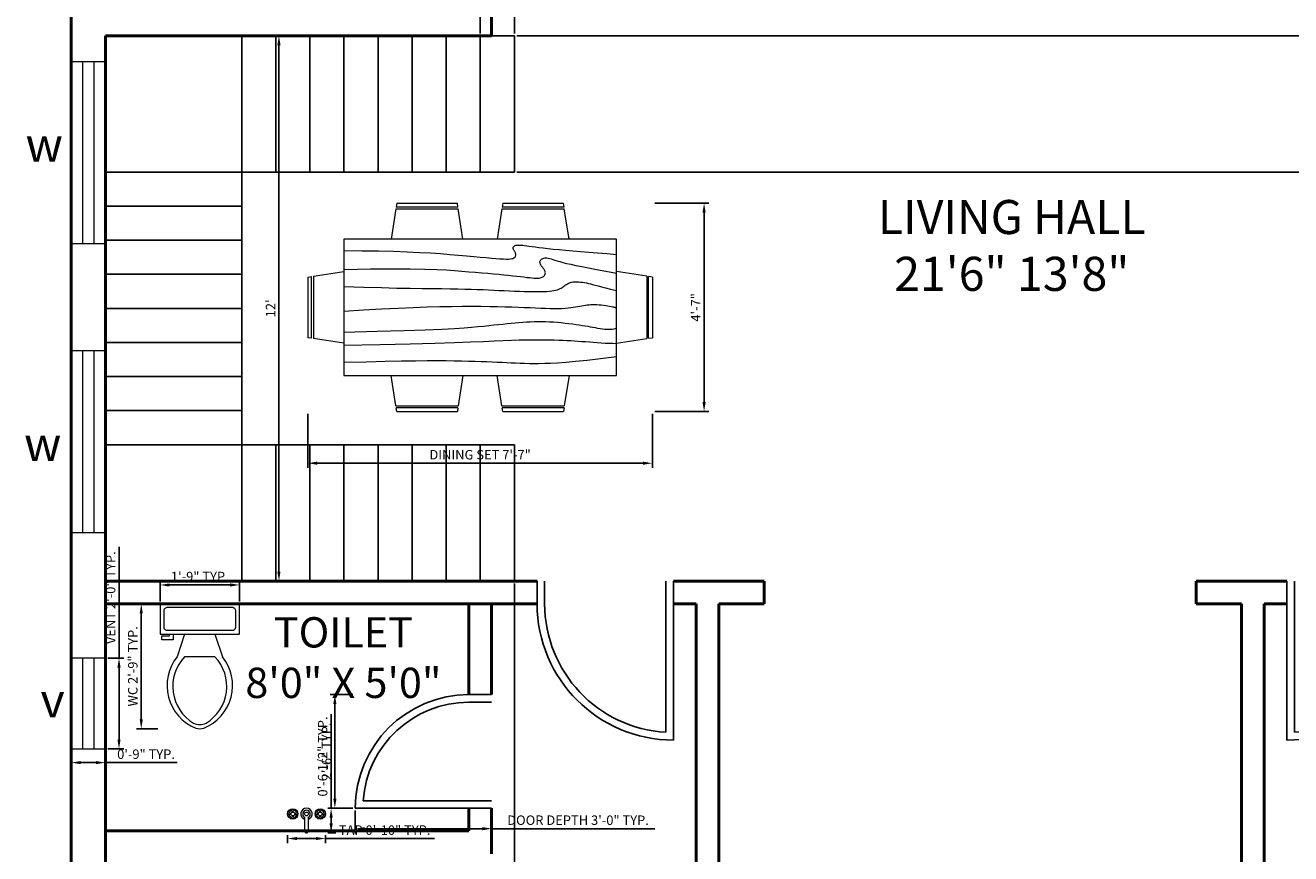
# Model space of a CAD drawing. Units: inches. Extents: x 1776 to 2338, y 1299 to 2099.
# Tile 2 of 4: x 1807 to 2141, y 1617 to 1836. Entities that reach past the tile are written whole.
import ezdxf

# ---------------------------------------------------------------- set-up
doc = ezdxf.new("R2010")
doc.units = ezdxf.units.IN
for name, color, linetype, lineweight in [('A-ANNO-DIMS', 2, 'Continuous', 18), ('A-ANNO-TEXT', 7, 'Continuous', 18), ('A-AREA-IDEN', 7, 'Continuous', 25), ('A-DOOR', 4, 'Continuous', 25), ('A-FLOR-FIXT', 9, 'Continuous', 18), ('A-FLOR-STRS', 7, 'Continuous', 25), ('A-FURN', 8, 'Continuous', 18), ('A-GLAZ', 4, 'Continuous', 18), ('A-WALL', 7, 'Continuous', 50)]:
    doc.layers.add(name, color=color, linetype=linetype, lineweight=lineweight)
doc.styles.get("Standard").update_dxf_attribs({"font": 'arial.ttf'})
doc.dimstyles.new('ISO-25', dxfattribs={"dimtxt": 2.5, "dimasz": 2.5, "dimexe": 1.25, "dimexo": 0.625, "dimtad": 1, "dimdec": 0, "dimlunit": 3, "dimtxsty": 'Standard', "dimcen": 2.5, "dimadec": 0, "dimazin": 0, "dimtfac": 1, "dimtdec": 0, "dimtmove": 0, "dimatfit": 3, "dimfxl": 1, "dimarcsym": 0})

# ---------------------------------------------------------------- blocks, each defined once
blk = doc.blocks.new('Dining Set - 36 x 72 in.')
for p, q in [((-22, 27.5), (-22.1562, 26.50042)), ((-22, 27.5), (-6, 27.5)), ((-5.8437, 26.49966), (-6, 27.5)), ((6, 27.5), (5.8438, 26.50042)), ((6, 27.5), (22, 27.5)), ((22.1563, 26.49966), (22, 27.5)), ((-22.2343, 26.00059), (-23.4847, 17.99762)), ((-22.2304, 26), (-5.7608, 26)), ((-5.8416, 26.5), (-22.1534, 26.5)), ((-4.5152, 17.99762), (-5.7655, 25.99926)), ((5.7657, 26.00059), (4.5153, 17.99762)), ((5.7696, 26), (22.2392, 26)), ((22.1584, 26.5), (5.8466, 26.5)), ((23.4848, 17.99762), (22.2345, 25.99926)), ((36, 18), (-36, 18)), ((-36, 18), (-36, -18)), ((36, -18), (36, 18)), ((-45.5, 8), (-44.5004, 8.15617)), ((-45.5, 8), (-45.5, -8)), ((-44.5, -8.15843), (-44.5, 8.15338)), ((-44.0006, 8.23428), (-35.9976, 9.48474)), ((-44, 8.23041), (-44, -8.23915)), ((44.0006, 8.23428), (35.9976, 9.48474)), ((44, 8.23041), (44, -8.23915)), ((44.5, -8.15843), (44.5, 8.15338)), ((45.5, 8), (44.5005, 8.15617)), ((45.5, 8), (45.5, -8)), ((-44.4997, -8.15631), (-45.5, -8)), ((-35.9976, -9.48476), (-43.9993, -8.2345)), ((35.9976, -9.48476), (43.9993, -8.2345)), ((44.4997, -8.15631), (45.5, -8)), ((-36, -18), (36, -18)), ((-22.2343, -26.0006), (-23.4847, -17.99762)), ((-4.5152, -17.99762), (-5.7655, -25.99928)), ((5.7657, -26.0006), (4.5153, -17.99762)), ((23.4848, -17.99762), (22.2345, -25.99928)), ((-22.2304, -26), (-5.7608, -26)), ((-22, -27.5), (-22.1562, -26.50044)), ((-5.8416, -26.5), (-22.1534, -26.5)), ((-5.8437, -26.49967), (-6, -27.5)), ((5.7696, -26), (22.2392, -26)), ((6, -27.5), (5.8438, -26.50044)), ((22.1584, -26.5), (5.8466, -26.5)), ((22.1563, -26.49967), (22, -27.5)), ((-22, -27.5), (-6, -27.5)), ((6, -27.5), (22, -27.5))]:
    blk.add_line(p, q)
for points in [[(-36, 15), (-31.1772, 14.97754), (-26.8079, 14.91406), (-22.8538, 14.81543), (-19.276, 14.6875), (-16.0362, 14.53613), (-13.0957, 14.36718), (-10.4159, 14.18652), (-7.9583, 14), (-5.6904, 13.81315), (-3.6035, 13.63021), (-1.6954, 13.45508), (0.0365, 13.29166), (1.5945, 13.14388), (2.9811, 13.01562), (4.1988, 12.9108), (5.25, 12.83333), (6.1393, 12.78613), (6.8802, 12.76823), (7.4883, 12.77767), (7.9792, 12.8125), (8.3685, 12.87077), (8.6719, 12.95052), (8.9049, 13.0498), (9.0833, 13.16666), (9.2205, 13.29899), (9.3216, 13.44401), (9.3895, 13.59879), (9.4271, 13.76041), (9.4373, 13.92594), (9.4232, 14.09245), (9.3875, 14.257), (9.3333, 14.41666), (9.2638, 14.56917), (9.1836, 14.71484), (9.0975, 14.85465), (9.0104, 14.98958), (8.9272, 15.1206), (8.8529, 15.2487), (8.7922, 15.37483), (8.75, 15.5), (8.7305, 15.62467), (8.7344, 15.74739), (8.7617, 15.86621), (8.8125, 15.97916), (8.8867, 16.08431), (8.9844, 16.17968), (9.1055, 16.26334), (9.25, 16.33333), (9.4189, 16.38802), (9.6172, 16.42708), (9.8506, 16.45052), (10.125, 16.45833), (10.4463, 16.45052), (10.8203, 16.42708), (11.2529, 16.38802), (11.75, 16.33333), (12.3184, 16.26318), (12.9694, 16.17838), (13.7151, 16.07991), (14.5677, 15.96875), (15.5395, 15.84586), (16.6426, 15.71224), (17.8893, 15.56884), (19.2917, 15.41666), (20.859, 15.25667), (22.5879, 15.08984), (24.4721, 14.91715), (26.5052, 14.73958), (28.6809, 14.5581), (30.9929, 14.3737), (33.4347, 14.18733), (36, 14)], [(-36, 10), (-28.9766, 10.14274), (-23.1725, 10.20442), (-18.4241, 10.19775), (-14.5677, 10.13541), (-11.4399, 10.03011), (-8.877, 9.89453), (-6.7154, 9.74137), (-4.7917, 9.58333), (-2.9698, 9.43082), (-1.2246, 9.28515), (0.4415, 9.14534), (2.026, 9.01041), (3.5266, 8.87939), (4.9408, 8.7513), (6.266, 8.62516), (7.5, 8.5), (8.6411, 8.37549), (9.6914, 8.2539), (10.6538, 8.13818), (11.5312, 8.03125), (12.3267, 7.93603), (13.043, 7.85547), (13.6831, 7.79248), (14.25, 7.75), (14.7471, 7.7303), (15.1797, 7.73307), (15.5537, 7.75732), (15.875, 7.80208), (16.1494, 7.86637), (16.3828, 7.94922), (16.5811, 8.04964), (16.75, 8.16666), (16.8944, 8.29915), (17.0143, 8.44531), (17.1089, 8.60319), (17.1771, 8.77083), (17.218, 8.94629), (17.2305, 9.1276), (17.2137, 9.31282), (17.1667, 9.5), (17.0895, 9.6875), (16.987, 9.875), (16.8649, 10.0625), (16.7292, 10.25), (16.5856, 10.4375), (16.4401, 10.625), (16.2985, 10.8125), (16.1667, 11), (16.05, 11.18733), (15.9518, 11.3737), (15.8752, 11.5581), (15.8229, 11.73958), (15.798, 11.91715), (15.8034, 12.08984), (15.842, 12.25667), (15.9167, 12.41666), (16.0295, 12.56836), (16.1784, 12.70833), (16.3605, 12.83268), (16.5729, 12.9375), (16.8127, 13.01888), (17.0768, 13.07291), (17.3625, 13.0957), (17.6667, 13.08333), (17.9894, 13.03312), (18.3418, 12.94726), (18.7382, 12.82918), (19.1927, 12.68229), (19.7195, 12.51001), (20.3327, 12.31575), (21.0465, 12.10294), (21.875, 11.875), (22.8357, 11.63354), (23.959, 11.37304), (25.2786, 11.08618), (26.8282, 10.76562), (28.6414, 10.40405), (30.752, 9.99414), (33.1936, 9.52856), (36, 9)], [(-36, 5.5), (-30.7157, 5.3348), (-26.069, 5.20963), (-21.9946, 5.11767), (-18.4271, 5.05208), (-15.3009, 5.00602), (-12.5508, 4.97265), (-10.1112, 4.94515), (-7.9167, 4.91666), (-5.909, 4.88167), (-4.0586, 4.83984), (-2.3429, 4.79215), (-0.7396, 4.73958), (0.7739, 4.6831), (2.22, 4.6237), (3.6213, 4.56233), (5, 4.5), (6.373, 4.43782), (7.7344, 4.3776), (9.0723, 4.32129), (10.375, 4.27083), (11.6309, 4.22819), (12.8281, 4.19531), (13.9551, 4.17415), (15, 4.16666), (15.954, 4.17448), (16.819, 4.19791), (17.6001, 4.23698), (18.3021, 4.29166), (18.9299, 4.36198), (19.4883, 4.44791), (19.9823, 4.54948), (20.4167, 4.66666), (20.7969, 4.79899), (21.1302, 4.94401), (21.4245, 5.09879), (21.6875, 5.26041), (21.9271, 5.42594), (22.1511, 5.59245), (22.3672, 5.757), (22.5834, 5.91666), (22.8065, 6.06868), (23.0404, 6.21093), (23.2879, 6.34147), (23.5521, 6.45833), (23.8358, 6.55957), (24.142, 6.64323), (24.4735, 6.70735), (24.8334, 6.75), (25.2235, 6.76969), (25.642, 6.76692), (26.0858, 6.74267), (26.5521, 6.69791), (27.0379, 6.63362), (27.5404, 6.55078), (28.0565, 6.45036), (28.5834, 6.33333), (29.1242, 6.19987), (29.7071, 6.04687), (30.3661, 5.87044), (31.1354, 5.66666), (32.0493, 5.43164), (33.142, 5.16146), (34.4475, 4.85221), (36, 4.5)], [(-36, -1), (-30.7915, -0.6591), (-26.0195, -0.38216), (-21.6519, -0.16284), (-17.6563, 0.00521), (-14.0005, 0.12833), (-10.6523, 0.21289), (-7.5796, 0.26522), (-4.75, 0.29166), (-2.134, 0.29793), (0.2878, 0.28711), (2.5317, 0.26163), (4.6146, 0.22396), (6.5529, 0.17651), (8.3633, 0.12174), (10.0623, 0.06209), (11.6667, 0), (13.1899, -0.06201), (14.6341, -0.1211), (15.9982, -0.17432), (17.2813, -0.21875), (18.4823, -0.25147), (19.6003, -0.26953), (20.6343, -0.27002), (21.5834, -0.25), (22.4481, -0.20768), (23.2357, -0.14584), (23.9549, -0.06836), (24.6146, 0.02083), (25.2235, 0.11784), (25.7904, 0.21875), (26.3241, 0.31966), (26.8334, 0.41666), (27.3265, 0.50618), (27.8099, 0.58593), (28.2894, 0.65397), (28.7709, 0.70833), (29.2601, 0.74707), (29.763, 0.76823), (30.2855, 0.76985), (30.8334, 0.75), (31.4088, 0.70784), (31.9994, 0.64713), (32.589, 0.57275), (33.1615, 0.48958), (33.7008, 0.4025), (34.1908, 0.3164), (34.6153, 0.23616), (34.9584, 0.16666), (35.2099, 0.11165), (35.3848, 0.07031), (35.504, 0.04069), (35.5886, 0.02083), (35.6594, 0.00879), (35.7377, 0.0026), (35.8442, 0.00032), (36, 0)], [(-36, -6.5), (-27.1843, -6.31267), (-20.084, -6.1263), (-14.469, -5.9419), (-10.1094, -5.76042), (-6.7752, -5.58285), (-4.2363, -5.41016), (-2.2629, -5.24333), (-0.625, -5.08334), (0.8708, -4.93099), (2.2715, -4.78646), (3.5872, -4.64974), (4.8281, -4.52084), (6.0046, -4.39974), (7.127, -4.28646), (8.2053, -4.18099), (9.25, -4.08334), (10.2705, -3.99382), (11.2734, -3.91407), (12.2647, -3.84603), (13.25, -3.79167), (14.2354, -3.75293), (15.2266, -3.73177), (16.2295, -3.73015), (17.25, -3.75), (18.2912, -3.79248), (19.3451, -3.85547), (20.4009, -3.93604), (21.4479, -4.03125), (22.4754, -4.13819), (23.4727, -4.25391), (24.4289, -4.37549), (25.3334, -4.5), (26.1785, -4.62492), (26.9694, -4.74935), (27.7145, -4.87281), (28.4219, -4.99479), (29.1, -5.11483), (29.7572, -5.23242), (30.4016, -5.34709), (31.0417, -5.45834), (31.6837, -5.56437), (32.3262, -5.65821), (32.9658, -5.73153), (33.599, -5.77604), (34.2224, -5.78345), (34.8327, -5.74545), (35.4264, -5.65373), (36, -5.5)], [(-36, -10), (-26.4022, -9.81299), (-18.4675, -9.62891), (-11.9839, -9.45069), (-6.7396, -9.28125), (-2.5226, -9.12354), (0.8789, -8.98047), (3.6769, -8.85498), (6.0833, -8.75), (8.2767, -8.66765), (10.3021, -8.60677), (12.1712, -8.56543), (13.8958, -8.54167), (15.4876, -8.53353), (16.9583, -8.53907), (18.3197, -8.55632), (19.5834, -8.58334), (20.7616, -8.61841), (21.8685, -8.66081), (22.9188, -8.71004), (23.9271, -8.76563), (24.9081, -8.82707), (25.8763, -8.89388), (26.8465, -8.96558), (27.8334, -9.04167), (28.8474, -9.12118), (29.8828, -9.20117), (30.93, -9.27824), (31.9792, -9.34896), (33.0205, -9.40991), (34.0443, -9.45768), (35.0407, -9.48885), (36, -9.5)], [(-36, -14.5), (-30.0881, -14.33513), (-25.0332, -14.21224), (-20.7312, -14.12647), (-17.0781, -14.07292), (-13.97, -14.04671), (-11.3027, -14.04297), (-8.9724, -14.05681), (-6.875, -14.08334), (-4.9224, -14.11833), (-3.0905, -14.16016), (-1.3709, -14.20785), (0.2448, -14.26042), (1.7647, -14.3169), (3.1973, -14.3763), (4.5507, -14.43767), (5.8333, -14.5), (7.0554, -14.5621), (8.235, -14.62175), (9.3922, -14.67652), (10.5469, -14.72396), (11.7192, -14.76164), (12.929, -14.78711), (14.1965, -14.79794), (15.5417, -14.79167), (16.9933, -14.76424), (18.6152, -14.70508), (20.4804, -14.60197), (22.6615, -14.44271), (25.2312, -14.21509), (28.2624, -13.9069), (31.8277, -13.50594), (36, -13)]]:
    blk.add_lwpolyline(points)
blk = doc.blocks.new('Toilet - top')
for p, q in [((9.5, -6), (9.5, -2)), ((-10, -8.5), (-8, -8.5)), ((-10, -9.5), (-10, -8.5)), ((-7, -9.5), (-10, -9.5)), ((-8, -8.5), (-8, -8)), ((-7, -8), (-7, -9.5)), ((-4, -8), (-6, -14)), ((4, -8), (6, -14)), ((4, -14), (-4, -14))]:
    blk.add_line(p, q)
blk.add_lwpolyline([(10.5, -8), (10.5, 0), (-10.5, 0), (-10.5, -8)], close=True)
for points in [[(-9.5, -2), (-9.5, -6)], [(8.5, -1), (-8.5, -1)], [(-8.5, -7), (8.5, -7)]]:
    blk.add_lwpolyline(points)
for centre, radius, start, end in [((-8.62, -1.88), 0.884, 81.8699, 188.1301), ((8.62, -1.88), 0.884, 351.8699, 98.1301), ((-8.62, -6.12), 0.884, 171.8699, 278.1301), ((8.62, -6.12), 0.884, 261.8699, 8.1301), ((3.52, -21.58), 12.17, 141.4691, 247.9714), ((4.2, -21.82), 11.33, 136.3677, 238.9468), ((-3.52, -21.58), 12.17, 292.0284, 38.5307), ((-4.2, -21.82), 11.33, 301.053, 43.6321), ((0, -27.88), 4, 245.7318, 294.2682), ((0, -29), 4, 254.8605, 285.1395)]:
    blk.add_arc(centre, radius, start, end)
blk = doc.blocks.new('Faucet - Bathroom top')
for p, q in [((-4.107, 0.125), (-4.375, 0.125)), ((-3.75, 0.4788), (-3.75, 0.75)), ((-3.5, 0.482), (-3.5, 0.75)), ((-3.1461, 0.125), (-2.875, 0.125)), ((3.143, 0.125), (2.875, 0.125)), ((3.5, 0.4788), (3.5, 0.75)), ((3.75, 0.482), (3.75, 0.75)), ((4.1039, 0.125), (4.375, 0.125)), ((-4.1039, -0.125), (-4.375, -0.125)), ((-3.75, -0.4821), (-3.75, -0.75)), ((-3.5, -0.4789), (-3.5, -0.75)), ((-3.143, -0.125), (-2.875, -0.125)), ((-0.5, -0.8639), (-0.5, -4.5)), ((0.5, -4.5), (0.5, -0.8631)), ((3.1461, -0.125), (2.875, -0.125)), ((3.5, -0.4821), (3.5, -0.75)), ((3.75, -0.4789), (3.75, -0.75)), ((4.107, -0.125), (4.375, -0.125))]:
    blk.add_line(p, q)
for centre, radius in [((-3.625, 0), 1.375), ((-4.625, 0), 0.2795), ((-3.625, 0), 0.5), ((-3.625, 1), 0.2795), ((-2.625, 0), 0.2795), ((0, 0), 0.5), ((3.625, 0), 1.375), ((2.625, 0), 0.2795), ((3.625, 0), 0.5), ((3.625, 1), 0.2795), ((4.625, 0), 0.2795), ((-3.625, -1), 0.2795), ((3.625, -1), 0.2795)]:
    blk.add_circle(centre, radius)
for centre, radius, start, end in [((-3.625, 0), 1, 105.2407, 164.2093), ((-3.625, 0), 1, 16.44125, 74.07887), ((0, 0), 1.5, 289.6514, 250.3603), ((0, 0), 1, 300.3431, 239.7554), ((3.625, 0), 1, 106.12, 164.0884), ((3.625, 0), 1, 16.23422, 73.90469), ((-3.625, 0), 1, 196.2342, 253.9047), ((-3.625, 0), 1, 286.12, 344.0884), ((3.625, 0), 1, 196.4413, 254.0789), ((3.625, 0), 1, 285.2407, 344.2093), ((0, -4.5), 0.5, 180, 0)]:
    blk.add_arc(centre, radius, start, end)
blk = doc.blocks.new('*D11')
at = {"layer": 'A-ANNO-DIMS', "color": 0, "lineweight": -2, "transparency": 16777216}
for p, q in [((1873.36, 1833.22), (1874.82, 1833.22)), ((1873.57, 1830.72), (1873.57, 1691.72)), ((1873.36, 1689.22), (1874.82, 1689.22))]:
    blk.add_line(p, q, dxfattribs=at)
at = {"layer": 'A-ANNO-DIMS', "color": 0, "transparency": 16777216}
for points in [[(1873.15, 1830.72), (1873.99, 1830.72), (1873.57, 1833.22)], [(1873.15, 1691.72), (1873.99, 1691.72), (1873.57, 1689.22)]]:
    blk.add_solid(points, dxfattribs=at)
at = {"layer": 'Defpoints', "color": 0, "transparency": 16777216}
for p in [(1872.74, 1833.22), (1872.74, 1689.22), (1873.57, 1689.22)]:
    blk.add_point(p, dxfattribs=at)
at = {"layer": 'A-ANNO-DIMS', "color": 0, "transparency": 16777216, "insert": (1871.69, 1761.22), "char_height": 2.5, "attachment_point": 5, "rotation": 90}
blk.add_mtext("12'", dxfattribs=at)
blk = doc.blocks.new('WIN-48IN')
for p, q in [((48, 9), (0, 9)), ((0, 9), (0, 0)), ((48, 0), (48, 9)), ((48, 6), (0, 6)), ((0, 3), (48, 3)), ((0, 0), (48, 0))]:
    blk.add_line(p, q)
blk = doc.blocks.new('VENT-24IN')
for p, q in [((9, 24), (0, 24)), ((0, 24), (0, 0)), ((3, 24), (3, 0)), ((6, 0), (6, 24)), ((9, 0), (9, 24)), ((0, 0), (9, 0))]:
    blk.add_line(p, q)
blk = doc.blocks.new('DOOR-36IN')
for p, q in [((36, 6), (36, 42)), ((34, 6), (34, 39.94)), ((0, 0), (0, 6)), ((2, 0), (2, 6)), ((34, 6), (34, 0)), ((36, 6), (36, 0))]:
    blk.add_line(p, q)
for radius, start in [(36, 90), (34, 93.3723)]:
    blk.add_arc((36, 6), radius, start, 180)
blk = doc.blocks.new('DOOR-30IN')
for p, q in [((0, 36), (0, 30)), ((2, 36), (2, 30)), ((28, 30), (28, 36)), ((30, 30), (30, 36)), ((28, 30), (28, 2.07)), ((30, 30), (30, 0))]:
    blk.add_line(p, q)
for radius, end in [(30, 270), (28, 265.904)]:
    blk.add_arc((30, 30), radius, 180, end)
blk = doc.blocks.new('*D22')
at = {"layer": 'A-ANNO-DIMS', "color": 0, "lineweight": -2, "transparency": 16777216}
for p, q in [((1831.34, 1668.87), (1831.34, 1698.27)), ((1828.36, 1668.87), (1832.59, 1668.87)), ((1831.34, 1647.37), (1831.34, 1666.37)), ((1828.36, 1644.87), (1832.59, 1644.87))]:
    blk.add_line(p, q, dxfattribs=at)
at = {"layer": 'A-ANNO-DIMS', "color": 0, "transparency": 16777216}
for points in [[(1830.92, 1666.37), (1831.76, 1666.37), (1831.34, 1668.87)], [(1830.92, 1647.37), (1831.76, 1647.37), (1831.34, 1644.87)]]:
    blk.add_solid(points, dxfattribs=at)
at = {"layer": 'Defpoints', "color": 0, "transparency": 16777216}
for p in [(1827.74, 1668.87), (1831.34, 1668.87), (1827.74, 1644.87)]:
    blk.add_point(p, dxfattribs=at)
at = {"layer": 'A-ANNO-DIMS', "color": 0, "transparency": 16777216, "insert": (1829.44, 1684.82), "char_height": 2.5, "attachment_point": 5, "rotation": 90}
blk.add_mtext('VENT 2\'-0" TYP.', dxfattribs=at)
blk = doc.blocks.new('*D23')
at = {"layer": 'A-ANNO-DIMS', "color": 0, "lineweight": -2, "transparency": 16777216}
for p, q in [((1818.74, 1644.24), (1818.74, 1640.02)), ((1827.74, 1644.24), (1827.74, 1640.02)), ((1821.24, 1641.27), (1825.24, 1641.27)), ((1827.74, 1641.27), (1846.73, 1641.27))]:
    blk.add_line(p, q, dxfattribs=at)
at = {"layer": 'A-ANNO-DIMS', "color": 0, "transparency": 16777216}
for points in [[(1821.24, 1641.69), (1821.24, 1640.85), (1818.74, 1641.27)], [(1825.24, 1641.69), (1825.24, 1640.85), (1827.74, 1641.27)]]:
    blk.add_solid(points, dxfattribs=at)
at = {"layer": 'Defpoints', "color": 0, "transparency": 16777216}
for p in [(1818.74, 1644.87), (1827.74, 1644.87), (1827.74, 1641.27)]:
    blk.add_point(p, dxfattribs=at)
at = {"layer": 'A-ANNO-DIMS', "color": 0, "transparency": 16777216, "insert": (1838.48, 1643.17), "char_height": 2.5, "attachment_point": 5}
blk.add_mtext('0\'-9" TYP.', dxfattribs=at)
blk = doc.blocks.new('*D26')
at = {"layer": 'A-ANNO-DIMS', "color": 0, "lineweight": -2, "transparency": 16777216}
for p, q in [((1841.55, 1683.22), (1835.96, 1683.22)), ((1837.21, 1652.67), (1837.21, 1680.72)), ((1841.55, 1650.17), (1835.96, 1650.17))]:
    blk.add_line(p, q, dxfattribs=at)
at = {"layer": 'A-ANNO-DIMS', "color": 0, "transparency": 16777216}
for points in [[(1836.8, 1680.72), (1837.63, 1680.72), (1837.21, 1683.22)], [(1836.8, 1652.67), (1837.63, 1652.67), (1837.21, 1650.17)]]:
    blk.add_solid(points, dxfattribs=at)
at = {"layer": 'Defpoints', "color": 0, "transparency": 16777216}
for p in [(1837.21, 1683.22), (1842.17, 1683.22), (1842.17, 1650.17)]:
    blk.add_point(p, dxfattribs=at)
at = {"layer": 'A-ANNO-DIMS', "color": 0, "transparency": 16777216, "insert": (1835.3, 1666.7), "char_height": 2.5, "attachment_point": 5, "rotation": 90}
blk.add_mtext('WC 2\'-9" TYP.', dxfattribs=at)
blk = doc.blocks.new('*D27')
at = {"layer": 'A-ANNO-DIMS', "color": 0, "lineweight": -2, "transparency": 16777216}
for p, q in [((1842.17, 1683.84), (1842.17, 1689.43)), ((1844.67, 1688.18), (1860.67, 1688.18)), ((1863.17, 1683.84), (1863.17, 1689.43))]:
    blk.add_line(p, q, dxfattribs=at)
at = {"layer": 'A-ANNO-DIMS', "color": 0, "transparency": 16777216}
for points in [[(1844.67, 1688.59), (1844.67, 1687.76), (1842.17, 1688.18)], [(1860.67, 1688.59), (1860.67, 1687.76), (1863.17, 1688.18)]]:
    blk.add_solid(points, dxfattribs=at)
at = {"layer": 'Defpoints', "color": 0, "transparency": 16777216}
for p in [(1863.17, 1688.18), (1842.17, 1683.22), (1863.17, 1683.22)]:
    blk.add_point(p, dxfattribs=at)
at = {"layer": 'A-ANNO-DIMS', "color": 0, "transparency": 16777216, "insert": (1852.67, 1690.08), "char_height": 2.5, "attachment_point": 5}
blk.add_mtext('1\'-9" TYP.', dxfattribs=at)
blk = doc.blocks.new('*D28')
at = {"layer": 'A-ANNO-DIMS', "color": 0, "lineweight": -2, "transparency": 16777216}
for p, q in [((1875.85, 1622.09), (1875.85, 1619.97)), ((1878.35, 1621.22), (1883.35, 1621.22)), ((1885.85, 1622.09), (1885.85, 1619.97)), ((1885.85, 1621.22), (1914.61, 1621.22))]:
    blk.add_line(p, q, dxfattribs=at)
at = {"layer": 'A-ANNO-DIMS', "color": 0, "transparency": 16777216}
for points in [[(1878.35, 1621.64), (1878.35, 1620.8), (1875.85, 1621.22)], [(1883.35, 1621.64), (1883.35, 1620.8), (1885.85, 1621.22)]]:
    blk.add_solid(points, dxfattribs=at)
at = {"layer": 'Defpoints', "color": 0, "transparency": 16777216}
for p in [(1875.85, 1622.72), (1885.85, 1622.72), (1885.85, 1621.22)]:
    blk.add_point(p, dxfattribs=at)
at = {"layer": 'A-ANNO-DIMS', "color": 0, "transparency": 16777216, "insert": (1901.48, 1623.12), "char_height": 2.5, "attachment_point": 5}
blk.add_mtext('TAP 0\'-10" TYP.', dxfattribs=at)
blk = doc.blocks.new('*D29')
at = {"layer": 'A-ANNO-DIMS', "color": 0, "lineweight": -2, "transparency": 16777216}
for p, q in [((1887.35, 1629.22), (1887.35, 1654.03)), ((1886.48, 1629.22), (1888.6, 1629.22)), ((1887.35, 1625.22), (1887.35, 1626.72)), ((1886.48, 1622.72), (1888.6, 1622.72))]:
    blk.add_line(p, q, dxfattribs=at)
at = {"layer": 'A-ANNO-DIMS', "color": 0, "transparency": 16777216}
for points in [[(1886.94, 1626.72), (1887.77, 1626.72), (1887.35, 1629.22)], [(1886.94, 1625.22), (1887.77, 1625.22), (1887.35, 1622.72)]]:
    blk.add_solid(points, dxfattribs=at)
at = {"layer": 'Defpoints', "color": 0, "transparency": 16777216}
for p in [(1885.85, 1629.22), (1887.35, 1629.22), (1885.85, 1622.72)]:
    blk.add_point(p, dxfattribs=at)
at = {"layer": 'A-ANNO-DIMS', "color": 0, "transparency": 16777216, "insert": (1885.44, 1642.88), "char_height": 2.5, "attachment_point": 5, "rotation": 90}
blk.add_mtext('0\'-6 1/2" TYP.', dxfattribs=at)
blk = doc.blocks.new('*D32')
at = {"layer": 'A-ANNO-DIMS', "color": 0, "lineweight": -2, "transparency": 16777216}
for p, q in [((1893.74, 1628.59), (1893.74, 1622.57)), ((1929.74, 1628.59), (1929.74, 1622.57)), ((1896.24, 1623.82), (1927.24, 1623.82)), ((1929.74, 1623.82), (1972.86, 1623.82))]:
    blk.add_line(p, q, dxfattribs=at)
at = {"layer": 'A-ANNO-DIMS', "color": 0, "transparency": 16777216}
for points in [[(1896.24, 1624.24), (1896.24, 1623.4), (1893.74, 1623.82)], [(1927.24, 1624.24), (1927.24, 1623.4), (1929.74, 1623.82)]]:
    blk.add_solid(points, dxfattribs=at)
at = {"layer": 'Defpoints', "color": 0, "transparency": 16777216}
for p in [(1893.74, 1629.22), (1929.74, 1629.22), (1929.74, 1623.82)]:
    blk.add_point(p, dxfattribs=at)
at = {"layer": 'A-ANNO-DIMS', "color": 0, "transparency": 16777216, "insert": (1952.55, 1625.74), "char_height": 2.5, "attachment_point": 5}
blk.add_mtext('DOOR DEPTH 3\'-0" TYP.', dxfattribs=at)
blk = doc.blocks.new('*D33')
at = {"layer": 'A-ANNO-DIMS', "color": 0, "lineweight": -2, "transparency": 16777216}
for p, q in [((1893.11, 1659.22), (1887.09, 1659.22)), ((1888.34, 1656.72), (1888.34, 1631.72)), ((1893.11, 1629.22), (1887.09, 1629.22))]:
    blk.add_line(p, q, dxfattribs=at)
at = {"layer": 'A-ANNO-DIMS', "color": 0, "transparency": 16777216}
for points in [[(1887.92, 1656.72), (1888.76, 1656.72), (1888.34, 1659.22)], [(1887.92, 1631.72), (1888.76, 1631.72), (1888.34, 1629.22)]]:
    blk.add_solid(points, dxfattribs=at)
at = {"layer": 'Defpoints', "color": 0, "transparency": 16777216}
for p in [(1893.74, 1659.22), (1888.34, 1629.22), (1893.74, 1629.22)]:
    blk.add_point(p, dxfattribs=at)
at = {"layer": 'A-ANNO-DIMS', "color": 0, "transparency": 16777216, "insert": (1886.44, 1644.22), "char_height": 2.5, "attachment_point": 5, "rotation": 90}
blk.add_mtext('2\'-6" TYP.', dxfattribs=at)
blk = doc.blocks.new('*D38')
at = {"layer": 'A-ANNO-DIMS', "color": 0, "lineweight": -2, "transparency": 16777216}
for p, q in [((1881.19, 1733.36), (1881.19, 1719.08)), ((1972.19, 1733.36), (1972.19, 1719.08)), ((1883.69, 1720.33), (1969.69, 1720.33))]:
    blk.add_line(p, q, dxfattribs=at)
at = {"layer": 'A-ANNO-DIMS', "color": 0, "transparency": 16777216}
for points in [[(1883.69, 1720.75), (1883.69, 1719.92), (1881.19, 1720.33)], [(1969.69, 1720.75), (1969.69, 1719.92), (1972.19, 1720.33)]]:
    blk.add_solid(points, dxfattribs=at)
at = {"layer": 'Defpoints', "color": 0, "transparency": 16777216}
for p in [(1881.19, 1733.98), (1972.19, 1733.98), (1972.19, 1720.33)]:
    blk.add_point(p, dxfattribs=at)
at = {"layer": 'A-ANNO-DIMS', "color": 0, "transparency": 16777216, "insert": (1926.69, 1722.25), "char_height": 2.5, "attachment_point": 5}
blk.add_mtext('DINING SET 7\'-7"', dxfattribs=at)
blk = doc.blocks.new('*D39')
at = {"layer": 'A-ANNO-DIMS', "color": 0, "lineweight": -2, "transparency": 16777216}
for p, q in [((1972.81, 1788.98), (1987.09, 1788.98)), ((1985.84, 1736.48), (1985.84, 1786.48)), ((1972.81, 1733.98), (1987.09, 1733.98))]:
    blk.add_line(p, q, dxfattribs=at)
at = {"layer": 'A-ANNO-DIMS', "color": 0, "transparency": 16777216}
for points in [[(1985.42, 1786.48), (1986.26, 1786.48), (1985.84, 1788.98)], [(1985.42, 1736.48), (1986.26, 1736.48), (1985.84, 1733.98)]]:
    blk.add_solid(points, dxfattribs=at)
at = {"layer": 'Defpoints', "color": 0, "transparency": 16777216}
for p in [(1972.19, 1788.98), (1985.84, 1788.98), (1972.19, 1733.98)]:
    blk.add_point(p, dxfattribs=at)
at = {"layer": 'A-ANNO-DIMS', "color": 0, "transparency": 16777216, "insert": (1983.96, 1761.48), "char_height": 2.5, "attachment_point": 5, "rotation": 90}
blk.add_mtext('4\'-7"', dxfattribs=at)
blk = doc.blocks.new('*D47')
at = {"layer": 'A-ANNO-DIMS', "color": 0, "lineweight": -2, "transparency": 16777216}
for p, q in [((1827.74, 1688.59), (1827.74, 1299.52)), ((1935.74, 1688.59), (1935.74, 1299.52)), ((1830.24, 1300.77), (1933.24, 1300.77))]:
    blk.add_line(p, q, dxfattribs=at)
at = {"layer": 'A-ANNO-DIMS', "color": 0, "transparency": 16777216}
for points in [[(1830.24, 1301.19), (1830.24, 1300.35), (1827.74, 1300.77)], [(1933.24, 1301.19), (1933.24, 1300.35), (1935.74, 1300.77)]]:
    blk.add_solid(points, dxfattribs=at)
at = {"layer": 'Defpoints', "color": 0, "transparency": 16777216}
for p in [(1827.74, 1689.22), (1935.74, 1689.22), (1935.74, 1300.77)]:
    blk.add_point(p, dxfattribs=at)
at = {"layer": 'A-ANNO-DIMS', "color": 0, "transparency": 16777216, "insert": (1881.74, 1302.67), "char_height": 2.5, "attachment_point": 5}
blk.add_mtext('9\'-0"', dxfattribs=at)
blk = doc.blocks.new('*D48')
at = {"layer": 'A-ANNO-DIMS', "color": 0, "lineweight": -2, "transparency": 16777216}
for p, q in [((1936.36, 1833.22), (2337.44, 1833.22)), ((2336.19, 1799.72), (2336.19, 1830.72)), ((1936.36, 1797.22), (2337.44, 1797.22))]:
    blk.add_line(p, q, dxfattribs=at)
at = {"layer": 'A-ANNO-DIMS', "color": 0, "transparency": 16777216}
for points in [[(2335.77, 1830.72), (2336.61, 1830.72), (2336.19, 1833.22)], [(2335.77, 1799.72), (2336.61, 1799.72), (2336.19, 1797.22)]]:
    blk.add_solid(points, dxfattribs=at)
at = {"layer": 'Defpoints', "color": 0, "transparency": 16777216}
for p in [(1935.74, 1833.22), (2336.19, 1833.22), (1935.74, 1797.22)]:
    blk.add_point(p, dxfattribs=at)
at = {"layer": 'A-ANNO-DIMS', "color": 0, "transparency": 16777216, "insert": (2334.29, 1815.22), "char_height": 2.5, "attachment_point": 5, "rotation": 90}
blk.add_mtext('3\'-0"', dxfattribs=at)
blk = doc.blocks.new('*D49')
at = {"layer": 'A-ANNO-DIMS', "color": 0, "lineweight": -2, "transparency": 16777216}
for p, q in [((1926.74, 1833.84), (1926.74, 2096.92)), ((1929.24, 2095.67), (1933.24, 2095.67)), ((1935.74, 1833.84), (1935.74, 2096.92))]:
    blk.add_line(p, q, dxfattribs=at)
at = {"layer": 'A-ANNO-DIMS', "color": 0, "transparency": 16777216}
for points in [[(1929.24, 2096.09), (1929.24, 2095.25), (1926.74, 2095.67)], [(1933.24, 2096.09), (1933.24, 2095.25), (1935.74, 2095.67)]]:
    blk.add_solid(points, dxfattribs=at)
at = {"layer": 'Defpoints', "color": 0, "transparency": 16777216}
for p in [(1935.74, 2095.67), (1926.74, 1833.22), (1935.74, 1833.22)]:
    blk.add_point(p, dxfattribs=at)
at = {"layer": 'A-ANNO-DIMS', "color": 0, "transparency": 16777216, "insert": (1931.24, 2097.57), "char_height": 2.5, "attachment_point": 5}
blk.add_mtext('0\'-9"', dxfattribs=at)

msp = doc.modelspace()

# ---------------------------------------------------------------- linework, layer by layer
at = {"layer": 'A-DOOR'}
msp.add_line((1975.74, 1647.27), (1975.74, 1647.22), dxfattribs=at)
at = {"layer": 'A-FLOR-STRS'}
for p, q in [((1863.74, 1689.22), (1863.74, 1833.22)), ((1863.74, 1689.22), (1863.74, 1833.22)), ((1872.74, 1797.22), (1872.74, 1833.22)), ((1881.74, 1797.22), (1881.74, 1833.22)), ((1890.74, 1797.22), (1890.74, 1833.22)), ((1899.74, 1797.22), (1899.74, 1833.22)), ((1908.74, 1797.22), (1908.74, 1833.22)), ((1917.74, 1797.22), (1917.74, 1833.22)), ((1926.74, 1797.22), (1926.74, 1833.22)), ((1935.74, 1833.22), (1929.74, 1833.22)), ((1935.74, 1797.22), (1935.74, 1833.22)), ((1827.74, 1797.22), (1929.74, 1797.22)), ((1929.74, 1797.22), (1935.74, 1797.22)), ((1827.74, 1788.22), (1863.74, 1788.22)), ((1827.74, 1779.22), (1863.74, 1779.22)), ((1827.74, 1770.22), (1863.74, 1770.22)), ((1827.74, 1761.22), (1863.74, 1761.22)), ((1827.74, 1752.22), (1863.74, 1752.22)), ((1827.74, 1743.22), (1863.74, 1743.22)), ((1827.74, 1734.22), (1863.74, 1734.22)), ((1827.74, 1725.22), (1929.74, 1725.22)), ((1872.74, 1689.22), (1872.74, 1725.22)), ((1881.74, 1689.22), (1881.74, 1725.22)), ((1890.74, 1689.22), (1890.74, 1725.22)), ((1899.74, 1689.22), (1899.74, 1725.22)), ((1908.74, 1689.22), (1908.74, 1725.22)), ((1917.74, 1689.22), (1917.74, 1725.22)), ((1926.74, 1689.22), (1926.74, 1725.22)), ((1929.74, 1725.22), (1935.74, 1725.22)), ((1935.74, 1689.22), (1935.74, 1725.22))]:
    msp.add_line(p, q, dxfattribs=at)
at = {"layer": 'A-WALL'}
for p, q in [((1818.74, 1338.22), (1818.74, 2058.22)), ((1929.74, 1833.22), (1929.74, 1899.22)), ((1827.74, 1833.22), (1929.74, 1833.22)), ((1827.74, 1473.22), (1827.74, 1833.22)), ((1827.74, 1689.22), (1929.74, 1689.22)), ((1929.74, 1689.22), (1941.74, 1689.22)), ((1977.74, 1689.22), (2001.74, 1689.22)), ((2001.74, 1683.22), (2001.74, 1689.22)), ((2115.74, 1683.22), (2115.74, 1689.22)), ((2115.74, 1689.22), (2139.74, 1689.22)), ((1827.74, 1683.22), (1929.74, 1683.22)), ((1923.74, 1659.22), (1923.74, 1683.22)), ((1929.74, 1683.22), (1941.74, 1683.22)), ((1929.74, 1659.22), (1929.74, 1683.22)), ((1983.74, 1683.22), (1977.74, 1683.22)), ((1977.74, 1683.22), (1983.74, 1683.22)), ((1983.74, 1473.22), (1983.74, 1683.22)), ((1989.74, 1473.22), (1989.74, 1683.22)), ((1989.74, 1683.22), (2001.74, 1683.22)), ((1989.74, 1683.22), (2001.74, 1683.22)), ((2127.74, 1683.22), (2115.74, 1683.22)), ((2115.74, 1683.22), (2127.74, 1683.22)), ((2127.74, 1683.22), (2127.74, 1473.22)), ((2133.74, 1683.22), (2133.74, 1473.22)), ((2133.74, 1683.22), (2139.74, 1683.22)), ((2133.74, 1683.22), (2139.74, 1683.22)), ((1923.74, 1623.22), (1923.74, 1629.22)), ((1923.74, 1623.22), (1923.74, 1629.22)), ((1929.74, 1617.22), (1929.74, 1629.22)), ((1827.74, 1623.22), (1923.74, 1623.22))]:
    msp.add_line(p, q, dxfattribs=at)

# ---------------------------------------------------------------- block references
at = {"layer": 'A-DOOR', "extrusion": (0, 0, -1), "zscale": -1, "rotation": 180}
msp.add_blockref('DOOR-36IN', (-1941.74, 1689.22), dxfattribs=at)
at = {"layer": 'A-DOOR'}
for name, p, rotation in [('DOOR-36IN', (2175.74, 1689.22), 180), ('DOOR-30IN', (1893.74, 1659.22), 269.9999999999997)]:
    msp.add_blockref(name, p, dxfattribs=dict(at, rotation=rotation))
at = {"layer": 'A-FLOR-FIXT'}
for name, p in [('Toilet - top', (1852.67, 1683.22)), ('Faucet - Bathroom top', (1880.85, 1627.72))]:
    msp.add_blockref(name, p, dxfattribs=at)
at = {"layer": 'A-FURN'}
msp.add_blockref('Dining Set - 36 x 72 in.', (1926.69, 1761.48), dxfattribs=at)
at = {"layer": 'A-GLAZ', "rotation": 269.999999999998}
for p in [(1818.74, 1826.34), (1818.74, 1750.01)]:
    msp.add_blockref('WIN-48IN', p, dxfattribs=at)
at = {"layer": 'A-GLAZ'}
msp.add_blockref('VENT-24IN', (1818.74, 1644.87), dxfattribs=at)

# ---------------------------------------------------------------- texts
at = {"layer": 'A-ANNO-TEXT', "char_height": 9, "attachment_point": 1}
for s, heights, insert in [('\\pxqc;w', [0], (1786.48, 1808.94)), ('\\pxqc;w', [0], (1786.08, 1729.96)), ('\\pxqc;v', [47.58], (1788.69, 1662.25))]:
    msp.add_mtext_dynamic_manual_height_columns(s, width=50.2204, gutter_width=12.5, heights=heights, dxfattribs=dict(at, insert=insert))
at = {"layer": 'A-AREA-IDEN', "attachment_point": 1}
for s, width, insert, char_height in [('\\pxqc;LIVING HALL\\P21\'6" 13\'8"', 108.1574, (2013.01, 1789.84), 9), ('\\pxqc;TOILET\\P8\'0" X 5\'0"', 54.6133, (1863.29, 1679.67), 8)]:
    msp.add_mtext_dynamic_manual_height_columns(s, width=width, gutter_width=12.5, heights=[0], dxfattribs=dict(at, insert=insert, char_height=char_height))

# ---------------------------------------------------------------- dimensions: what is measured, and where the dimension line sits
at = {"layer": 'A-ANNO-DIMS'}
for base, p1, p2, picture, middle in [((1935.74, 2095.67), (1926.74, 1833.22), (1935.74, 1833.22), '*D49', (1931.24, 2097.57)), ((1935.74, 1300.77), (1827.74, 1689.22), (1935.74, 1689.22), '*D47', (1881.74, 1302.67))]:
    dim = msp.add_linear_dim(base=base, p1=p1, p2=p2, dimstyle='ISO-25', override={"dimdec": 1, "dimlfac": 1, "dimrnd": 0, "dimzin": 1, "dimdsep": 46, "dimlunit": 4, "dimfrac": 2}, dxfattribs=at)
    dim.commit()
    dim.dimension.update_dxf_attribs({"geometry": picture, "text_midpoint": middle})
for base, p1, p2, override, picture, middle in [((1873.57, 1689.22), (1872.74, 1833.22), (1872.74, 1689.22), {"dimclrd": 0, "dimclre": 0, "dimclrt": 0}, '*D11', (1871.69, 1761.22)), ((2336.19, 1833.22), (1935.74, 1797.22), (1935.74, 1833.22), {"dimdec": 1, "dimlfac": 1, "dimrnd": 0, "dimzin": 1, "dimdsep": 46, "dimlunit": 4, "dimfrac": 2}, '*D48', (2334.29, 1815.22)), ((1985.84, 1788.98), (1972.19, 1733.98), (1972.19, 1788.98), {"dimdec": 1, "dimlfac": 1, "dimrnd": 0, "dimzin": 1, "dimdsep": 46, "dimlunit": 4, "dimfrac": 2}, '*D39', (1983.96, 1761.48))]:
    dim = msp.add_linear_dim(base=base, p1=p1, p2=p2, angle=90, dimstyle='ISO-25', override=override, dxfattribs=at)
    dim.commit()
    dim.dimension.update_dxf_attribs({"geometry": picture, "text_midpoint": middle})
for base, p1, p2, text, picture, middle in [((1972.19, 1720.33), (1881.19, 1733.98), (1972.19, 1733.98), 'DINING SET <>', '*D38', (1926.69, 1722.25)), ((1863.17, 1688.18), (1842.17, 1683.22), (1863.17, 1683.22), '<> TYP.', '*D27', (1852.67, 1690.08)), ((1827.74, 1641.27), (1818.74, 1644.87), (1827.74, 1644.87), '<> TYP.', '*D23', (1838.48, 1643.17)), ((1929.74, 1623.82), (1893.74, 1629.22), (1929.74, 1629.22), 'DOOR DEPTH <> TYP.', '*D32', (1952.55, 1625.74)), ((1885.85, 1621.22), (1875.85, 1622.72), (1885.85, 1622.72), 'TAP <> TYP.', '*D28', (1901.48, 1623.12))]:
    dim = msp.add_linear_dim(base=base, p1=p1, p2=p2, text=text, dimstyle='ISO-25', override={"dimdec": 1, "dimlfac": 1, "dimrnd": 0, "dimzin": 1, "dimdsep": 46, "dimlunit": 4, "dimfrac": 2}, dxfattribs=at)
    dim.commit()
    dim.dimension.update_dxf_attribs({"geometry": picture, "text_midpoint": middle})
for base, p1, p2, angle, text, picture, middle in [((1831.34, 1668.87), (1827.74, 1644.87), (1827.74, 1668.87), 90, 'VENT <> TYP.', '*D22', (1829.44, 1684.82)), ((1837.2141, 1683.2187), (1842.171, 1650.1725), (1842.171, 1683.2187), 90, 'WC <> TYP.', '*D26', (1835.2964, 1666.6956)), ((1888.34, 1629.22), (1893.74, 1659.22), (1893.74, 1629.22), 270, '<> TYP.', '*D33', (1886.44, 1644.22)), ((1887.35, 1629.22), (1885.85, 1622.72), (1885.85, 1629.22), 90, '<> TYP.', '*D29', (1885.44, 1642.88))]:
    dim = msp.add_linear_dim(base=base, p1=p1, p2=p2, angle=angle, text=text, dimstyle='ISO-25', override={"dimdec": 1, "dimlfac": 1, "dimrnd": 0, "dimzin": 1, "dimdsep": 46, "dimlunit": 4, "dimfrac": 2}, dxfattribs=at)
    dim.commit()
    dim.dimension.update_dxf_attribs({"geometry": picture, "text_midpoint": middle})

doc.saveas('drawing.dxf')
